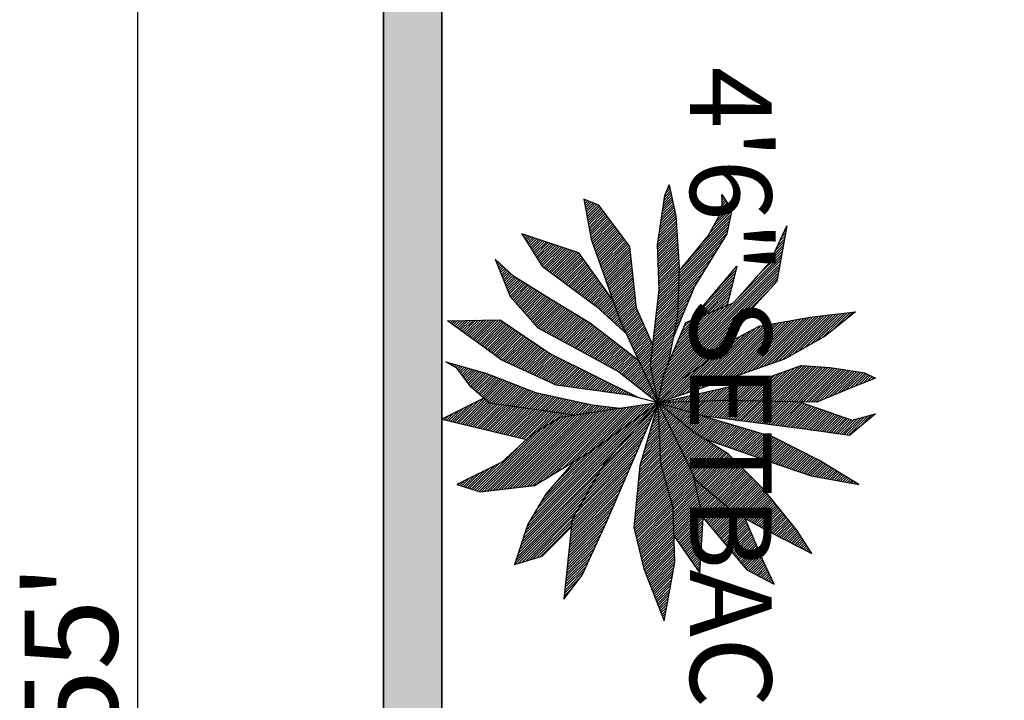
# Model space of a CAD drawing. Units: inches. Extents: x 3008 to 4088, y 1255 to 2137.
# Tile 6 of 30: x 3008 to 3093, y 1670 to 1728. Entities that reach past the tile are written whole.
import ezdxf

# ---------------------------------------------------------------- set-up
doc = ezdxf.new("R2010")
doc.units = ezdxf.units.IN
for name, color, linetype, lineweight in [('A-ANNO-DIMS', 2, 'Continuous', 18), ('A-ANNO-TEXT', 7, 'Continuous', 18), ('C-PROP', 1, 'Continuous', 35), ('C-PROP-PATT', 9, 'Continuous', 13), ('L-PLNT', 3, 'Continuous', 13), ('vfolhas', 114, 'Continuous', 5)]:
    doc.layers.add(name, color=color, linetype=linetype, lineweight=lineweight)
for name, color, linetype in [('vfolha', 72, 'Continuous'), ('vfolha2', 110, 'Continuous'), ('vfolhas2', 102, 'Continuous')]:
    doc.layers.add(name, color=color, linetype=linetype)
doc.styles.get("Standard").update_dxf_attribs({"font": 'arial.ttf'})
doc.dimstyles.new('ISO-25', dxfattribs={"dimtxt": 8, "dimasz": 2.5, "dimexe": 1.25, "dimexo": 0.625, "dimtad": 1, "dimdec": 1, "dimlunit": 3, "dimtxsty": 'Standard', "dimcen": 2.5, "dimadec": 0, "dimazin": 0, "dimtfac": 1, "dimtdec": 1, "dimtmove": 0, "dimatfit": 3, "dimfxl": 1, "dimarcsym": 0})
pattern_1 = [(45, (-2446.513311328918, 50.98607575111775), (-0.0044194173824159, 0.0044194173824159), [])]

# ---------------------------------------------------------------- blocks, each defined once
blk = doc.blocks.new('*D2')
at = {"layer": 'A-ANNO-DIMS', "color": 0, "lineweight": -2, "transparency": 16777216}
for p, q in [((3039.040660450281, 2003.966263701819), (3017.259837783714, 2003.966263701819)), ((3018.509837783714, 2001.466263701819), (3018.509837783714, 1346.466263701818)), ((3039.040660450281, 1343.966263701819), (3017.259837783714, 1343.966263701819))]:
    blk.add_line(p, q, dxfattribs=at)
at = {"layer": 'A-ANNO-DIMS', "color": 0, "transparency": 16777216}
for points in [[(3018.093171117048, 2001.466263701819), (3018.926504450381, 2001.466263701819), (3018.509837783714, 2003.966263701819)], [(3018.093171117048, 1346.466263701818), (3018.926504450381, 1346.466263701818), (3018.509837783714, 1343.966263701819)]]:
    blk.add_solid(points, dxfattribs=at)
at = {"layer": 'Defpoints', "color": 0, "transparency": 16777216}
for p in [(3039.665660450281, 2003.966263701819), (3018.509837783714, 1343.966263701819), (3039.665660450281, 1343.966263701819)]:
    blk.add_point(p, dxfattribs=at)
at = {"layer": 'A-ANNO-DIMS', "color": 0, "transparency": 16777216, "insert": (3013.816624959703, 1673.966263701817), "char_height": 8, "attachment_point": 5, "rotation": 90}
blk.add_mtext("55'", dxfattribs=at)
blk = doc.blocks.new('arbusto_PB_verde_grande')
at = {"layer": 'vfolha2'}
h = blk.add_hatch(dxfattribs=at)
h.set_pattern_fill('ANSI31', color=256, scale=0.05, style=0)
h.set_pattern_definition(pattern_1)
h.paths.add_polyline_path([(0.0294372067806137, 0.3565111995000905), (0.0002757213374309, 0.0904824516967153), (0.0262526469860234, -0.0393387531877068), (0.0469981892233875, 0.0623276281037022), (0.061889225542192, 0.09730735603225), (0.0937206571093441, 0.2657290609879511), (0.0995529541983444, 0.4347266728475463), (0.0878883600207985, 0.6131321160052893), (0.0644950804894791, 0.7226612468122938), (0.0498822921795466, 0.6850985919211043), (0.0236049096920681, 0.5129421461949732)])
h.paths.add_polyline_path([(0.3010556140521033, 0.4378855067140819), (0.1422506528203503, 0.2487134447506216), (0.266852050905866, 0.3002231891941697)])
h.paths.add_polyline_path([(0.3799518526907661, 0.2281664060967614), (0.23696550788001, 0.1519283823737274), (0.1842814899255529, 0.0936412855632796), (0.1112175483754357, 0.0435806358088371), (0.0262526469860234, -0.0393387531877068), (0.2806105286531701, 0.046670799373942), (0.368287258513679, 0.0779844568334922), (0.4675644913741336, 0.1123882778581162), (0.6106800891643901, 0.1937625850721077), (0.7158537102905315, 0.2782270558511755), (0.5581253241898877, 0.2594800635563387)])
h.paths.add_polyline_path([(0.5610094271460472, -0.2944145879103532), (0.7275183044680773, -0.3257282453699304), (0.5902350037659124, -0.2411951042894033), (0.4296225147095642, -0.1598207970754118), (0.0262526469860234, -0.0393387531877068), (0.1492236162166875, -0.1410738047805182), (0.188384525729089, -0.1660430415962635), (0.4150097263996438, -0.2443539381559163)])
h.paths.add_polyline_path([(-0.2742908800664451, -0.4477553710401593), (-0.3035164566863102, -0.7262821137067874), (-0.2392330063575799, -0.6417489726262603), (-0.1545685618070526, -0.4571632023383334), (0.0262526469860234, -0.0393387531877068), (-0.1632849618517582, -0.253761769454087)])
h.paths.add_polyline_path([(-0.5196319048504564, -0.2474441017210154), (-0.6773602909511, -0.3257282453699304), (-0.595579949356278, -0.3507242350964077), (-0.4057418836796105, -0.3288184089350068), (-0.2100715209143972, -0.2099501171312569), (0.0262526469860234, -0.0393387531877067), (-0.1487362647185048, -0.0659484949981665), (-0.3151810508638561, -0.0910131550261326), (-0.4145223749009972, -0.1504816360786947)])
h.paths.add_polyline_path([(-0.525464201939002, 0.2500722322581623), (-0.7094699705271239, 0.2469820686930859), (-0.5196319048504563, 0.1092981142930683), (-0.3297938391737886, 0.0216748096474362), (-0.0756723231683907, -0.012797681678677), (-0.0423442733277238, -0.0214762434946634), (-0.3502389245722667, 0.1312039404544406)])
h = blk.add_hatch(dxfattribs=at)
h.set_pattern_fill('ANSI31', color=256, scale=0.05, style=0)
h.set_pattern_definition(pattern_1)
h.paths.add_polyline_path([(-0.1896264355159187, 0.2970427184474999), (-0.0855343194014637, 0.2019191130931916), (-0.107846093921097, 0.2500722322581624), (-0.1320163779363008, 0.3186521089488384), (-0.2509616917118081, 0.4847873226019602), (-0.4495161574327255, 0.5505048010861913), (-0.3794645011925866, 0.437885506714082)])
h.paths.add_polyline_path([(0.0791078687994116, -0.4071025525838933), (0.0821399376597343, -0.5063128890747639), (0.1725528045713247, -0.635499975194648), (0.1842814899255529, -0.4415063736085472), (0.1490398072856009, -0.2917737067340336), (0.0262526469860234, -0.0393387531877068), (0.035269503869614, -0.253761769454087)])
at = {"layer": 'vfolhas'}
h = blk.add_hatch(dxfattribs=at)
h.set_pattern_fill('ANSI31', color=256, scale=0.05, style=0)
h.set_pattern_definition(pattern_1)
h.paths.add_polyline_path([(-0.0727882202122316, 0.506693148763361), (-0.180845944294532, 0.6506261005950194), (-0.2334007092690343, 0.6725319267564202), (-0.2071233267820105, 0.5317578087913261), (-0.1078460939210969, 0.2500722322581621), (0.0262526469860234, -0.0393387531877067), (0.0002757213374309, 0.0904824516967153), (0.0081597239746827, 0.1624051030085992), (-0.049394940681367, 0.2907937210158594)])
h.paths.add_polyline_path([(0.0990202003692698, 0.4192895091625076), (0.0937206571093441, 0.265729060987951), (0.0790571961243617, 0.1881439516147792), (0.1550559133052331, 0.3690091943633431), (0.2660618315199201, 0.5505048010861912), (0.2835587227860117, 0.6350379421667186), (0.2485008490776011, 0.6881887554862091), (0.2514490432099876, 0.6350379421667185), (0.2017783811911896, 0.5442558036545505)])
h.paths.add_polyline_path([(0.1229462337296639, 0.2407330712614737), (0.0469981892233875, 0.0623276281037022), (0.0262526469860234, -0.0393387531877067), (0.1112175483754356, 0.0435806358088371), (0.1842814899255529, 0.0936412855632796), (0.274778231564625, 0.1937625850721078), (0.3215006994505813, 0.2532310661246982), (0.4412871088866554, 0.3846660230931321), (0.4763449825955206, 0.5786596246792043), (0.4178938293553358, 0.4534736651424111), (0.289391019875012, 0.3095407133107528)])
h.paths.add_polyline_path([(0.581454512544525, -0.0377936714051543), (0.7070732190691449, 0.0153571419143647), (0.7859053665311252, 0.0466707993739419), (0.7479633898665554, 0.065486461970238), (0.6281769804304814, 0.0842334542651031), (0.5259515534371815, 0.0904824516967153), (0.3974487439568576, 0.0435806358088371), (0.0262526469860234, -0.0393387531877068), (0.2572813402989879, -0.0315446739735137), (0.4383389147538148, -0.034703507840078)])
h.paths.add_polyline_path([(0.5202160126333567, -0.0364714047610799), (0.438338914753814, -0.0347035078400779), (0.2572813402989879, -0.0315446739735137), (0.0262526469860234, -0.0393387531877068), (0.1796378832922042, -0.0851531985667382), (0.5376802387914114, -0.131665973482399), (0.6954086248920532, -0.1535717996437711), (0.785905366531125, -0.0785151601628513), (0.7041250249367578, -0.1004209863242522)])
h.paths.add_polyline_path([(0.2718941286089205, -0.2192892781280023), (0.1492236162166876, -0.1410738047805182), (0.0262526469860234, -0.0393387531877068), (0.1579400162613921, -0.3100714166401416), (0.2952233169635576, -0.4258495448787585), (0.4178938293553374, -0.4915670233629906), (0.5639576212784335, -0.5666923331453404), (0.5114028563039311, -0.4853180259313772), (0.3945646410006986, -0.3413850740996906)])
h.paths.add_polyline_path([(-0.0581754319022991, -0.4759101946332009), (-0.0231175581938885, -0.6198431464648595), (0.0469981892233875, -0.8013387531877071), (0.0849401658879572, -0.59793732030343), (0.0791078687994116, -0.4071025525838934), (0.035269503869614, -0.2537617694540871), (0.0262526469860234, -0.0393387531877068), (-0.037730346503821, -0.2600107668856992)])
h.paths.add_polyline_path([(-0.242181200490421, 0.1405431014511577), (-0.1107301968772561, 0.0685766255353144), (0.0262526469860234, -0.0393387531877067), (-0.0423455789620989, 0.1087094688700612), (-0.210071520914397, 0.2375742373949095), (-0.3648517128822022, 0.331446539472184), (-0.4787417340530456, 0.4034130153879689), (-0.5430251843817758, 0.4628814964405878), (-0.4904063282301365, 0.3314465394721821), (-0.394077289502519, 0.2219174086651207)])
h = blk.add_hatch(dxfattribs=at)
h.set_pattern_fill('ANSI31', color=256, scale=0.05, style=0)
h.set_pattern_definition(pattern_1)
h.paths.add_polyline_path([(-0.5721866698249584, 0.0623276281037022), (-0.7153022676152148, 0.1029804465599682), (-0.6773602909511, 0.0810746203985957), (-0.6276896289323022, 0.0153571419143646), (-0.5634702697802538, -0.0409525052716901), (-0.2646143236521083, -0.0833983906610745), (-0.1487362647185102, -0.0659484949981675), (-0.1015103002611421, -0.0587670644222552), (-0.2041751326491691, -0.0472015027033024), (-0.402793689546769, -0.0033898503805005)])
h.paths.add_polyline_path([(-0.5634702697802538, -0.0409525052716901), (-0.5827900422908869, -0.0240122930342424), (-0.7299150559256019, -0.0972621524577449), (-0.4334045373284922, -0.167900237669902), (-0.4145223749009971, -0.1504816360786947), (-0.3151810508638562, -0.0910131550261326), (-0.2646143236521083, -0.0833983906610745)])
h.paths.add_polyline_path([(-0.2769047876357005, -0.472666536023008), (-0.2742908800664452, -0.4477553710401595), (-0.1632849618517582, -0.253761769454087), (0.0262526469860233, -0.0393387531877068), (-0.2100715209143968, -0.2099501171312565), (-0.2672033595069225, -0.2446572846610163), (-0.3648517128821993, -0.35697323252802), (-0.4290710720342474, -0.4634121997699482), (-0.4758576310968862, -0.6042549880365016), (-0.3794645011925866, -0.576031494142029)])
h = blk.add_hatch(dxfattribs=at)
h.set_pattern_fill('ANSI31', color=256, scale=0.05, style=0)
h.set_pattern_definition(pattern_1)
h.paths.add_polyline_path([(0.3361134877609686, -0.6230019803313951), (0.4325066176652684, -0.6730626300858094), (0.3945646410006983, -0.5948471567383816), (0.3303002489141496, -0.4446410822727964), (0.2952233169635579, -0.4258495448787589), (0.1579400162613922, -0.3100714166401417), (0.1490398072856009, -0.2917737067340336), (0.184281489925553, -0.4415063736085473)])
at = {"layer": 'vfolha'}
for p, q in [((0.0262526469860234, -0.0393387531877068), (-0.148736264718508, -0.0659484949981675)), ((0.0262526469860234, -0.0393387531877068), (-0.037730346503821, -0.2600107668856992)), ((0.035269503869614, -0.253761769454087), (0.0262526469860234, -0.0393387531877068)), ((0.5202160126332558, -0.0364714047610448), (0.7041250249367579, -0.1004209863242522)), ((0.5376802387914097, -0.1316659734823986), (0.1796378832919174, -0.0851531985667009)), ((0.7859053665311251, -0.0785151601628513), (0.6954086248920534, -0.1535717996437711)), ((0.7041250249367579, -0.1004209863242522), (0.7859053665311251, -0.0785151601628513)), ((0.6954086248920534, -0.1535717996437711), (0.5376802387914097, -0.1316659734823986)), ((0.3945646410006986, -0.3413850740996906), (0.2718941286089205, -0.2192892781280022)), ((-0.2672033595067376, -0.2446572846608035), (-0.3648517128821993, -0.3569732325280199)), ((-0.037730346503821, -0.2600107668856992), (-0.0581754319022991, -0.475910194633201)), ((0.0791078687994116, -0.4071025525838934), (0.035269503869614, -0.253761769454087)), ((0.1579400162613922, -0.3100714166401417), (0.2952233169635576, -0.4258495448787585)), ((0.5114028563039313, -0.4853180259313774), (0.3945646410006986, -0.3413850740996906)), ((0.0849401658879572, -0.59793732030343), (0.0791078687994116, -0.4071025525838934)), ((0.2952233169635576, -0.4258495448787585), (0.4178938293553358, -0.4915670233629897)), ((0.4178938293553358, -0.4915670233629897), (0.5639576212784334, -0.5666923331453404)), ((0.5639576212784334, -0.5666923331453404), (0.5114028563039313, -0.4853180259313774)), ((0.0469981892233875, -0.8013387531877071), (0.0849401658879572, -0.59793732030343)), ((-0.0231175581938885, -0.6198431464648593), (0.0469981892233875, -0.8013387531877071))]:
    blk.add_line(p, q, dxfattribs=at)
at = {"layer": 'vfolha2'}
for p, q in [((0.0498822921795466, 0.6850985919211042), (0.0644950804894791, 0.7226612468122938)), ((0.0644950804894791, 0.7226612468122938), (0.0878883600207985, 0.6131321160052892)), ((0.0236049096920681, 0.5129421461949732), (0.0498822921795466, 0.6850985919211042)), ((0.0878883600207985, 0.6131321160052892), (0.0995529541983444, 0.4347266728475461)), ((-0.4495161574327256, 0.5505048010861913), (-0.3794645011925866, 0.4378855067140819)), ((-0.250961691711808, 0.4847873226019602), (-0.4495161574327256, 0.5505048010861913)), ((-0.1320163779364236, 0.31865210894901), (-0.250961691711808, 0.4847873226019602)), ((0.0294372067806137, 0.3565111995000905), (0.0236049096920681, 0.5129421461949732)), ((-0.3794645011925866, 0.4378855067140819), (-0.1896264355159189, 0.2970427184475)), ((0.0995529541983444, 0.4347266728475461), (0.0937206571093441, 0.265729060987951)), ((0.143391319128142, 0.2500722322581623), (0.3010556140521032, 0.4378855067140819)), ((0.3010556140521032, 0.4378855067140819), (0.2660618315199201, 0.2970427184475)), ((0.0002757213374309, 0.0904824516967153), (0.0294372067806137, 0.3565111995000905)), ((-0.1896264355159189, 0.2970427184475), (-0.0822034303200496, 0.1988752113042125)), ((0.5581253241898878, 0.2594800635563388), (0.7158537102905314, 0.2782270558511755)), ((0.7158537102905314, 0.2782270558511755), (0.61068008916439, 0.1937625850721076)), ((-0.7094699705271239, 0.2469820686930859), (-0.5254642019390019, 0.2500722322581623)), ((-0.5196319048504563, 0.1092981142930682), (-0.7094699705271239, 0.2469820686930859)), ((-0.5254642019390019, 0.2500722322581623), (-0.3502389245722668, 0.1312039404544407)), ((0.3799518526907661, 0.2281664060967614), (0.5581253241898878, 0.2594800635563388)), ((0.2369655078796597, 0.1519283823735407), (0.3799518526907661, 0.2281664060967614)), ((0.61068008916439, 0.1937625850721076), (0.4675644913741337, 0.1123882778581162)), ((-0.3297938391737887, 0.0216748096474362), (-0.5196319048504563, 0.1092981142930682)), ((-0.3502389245722668, 0.1312039404544407), (-0.0423442733276431, -0.0214762434947034)), ((0.0262526469860234, -0.0393387531877068), (0.0002757213374309, 0.0904824516967153)), ((0.3682872585136749, 0.0779844568334909), (0.2806105286531704, 0.0466707993739419)), ((0.2806105286531704, 0.0466707993739419), (0.0262526469860234, -0.0393387531877068)), ((-0.0756723231683907, -0.012797681678677), (-0.3297938391737887, 0.0216748096474362)), ((-0.148736264718508, -0.0659484949981675), (-0.3151810508638562, -0.0910131550261326)), ((-0.2100715209143971, -0.2099501171312568), (0.0262526469860234, -0.0393387531877068)), ((0.0262526469860234, -0.0393387531877068), (-0.1632849618517582, -0.253761769454087)), ((-0.1545685618070536, -0.4571632023383359), (0.0262526469860234, -0.0393387531877068)), ((0.4296225147095641, -0.1598207970754117), (0.0262526469860234, -0.0393387531877068)), ((0.0262526469860234, -0.0393387531877068), (0.1579400162613922, -0.3100714166401417)), ((-0.3151810508638562, -0.0910131550261326), (-0.4145223749009972, -0.1504816360786947)), ((-0.4145223749009972, -0.1504816360786947), (-0.5196319048504563, -0.2474441017210154)), ((0.1883845257293899, -0.1660430415963674), (0.4150097263996316, -0.2443539381559105)), ((0.5902350037659119, -0.2411951042894032), (0.4296225147095641, -0.1598207970754117)), ((-0.4057418836796103, -0.3288184089350068), (-0.2100715209143971, -0.2099501171312568)), ((-0.5196319048504563, -0.2474441017210154), (-0.6773602909511, -0.3257282453699304)), ((-0.1632849618517582, -0.253761769454087), (-0.2742908800664452, -0.4477553710401594)), ((0.4150097263996316, -0.2443539381559105), (0.5610094271460468, -0.294414587910353)), ((0.7275183044680773, -0.3257282453699304), (0.5902350037659119, -0.2411951042894032)), ((0.1842814899255529, -0.4415063736085472), (0.1490398072865275, -0.2917737067379704)), ((0.5610094271460468, -0.294414587910353), (0.7275183044680773, -0.3257282453699304)), ((-0.6773602909511, -0.3257282453699304), (-0.5955799493562779, -0.3507242350964077)), ((-0.5955799493562779, -0.3507242350964077), (-0.4057418836796103, -0.3288184089350068)), ((0.1725528045713247, -0.635499975194648), (0.1842814899255529, -0.4415063736085472)), ((-0.2742908800664452, -0.4477553710401594), (-0.3035164566863102, -0.7262821137067875)), ((0.0821399376596048, -0.5063128890745788), (0.1725528045713247, -0.635499975194648)), ((-0.3035164566863102, -0.7262821137067875), (-0.2392330063575798, -0.6417489726262602))]:
    blk.add_line(p, q, dxfattribs=at)
at = {"layer": 'vfolhas2'}
for p, q in [((-0.2334007092690342, 0.6725319267564203), (-0.2071233267820105, 0.5317578087913262)), ((-0.180845944294532, 0.6506261005950194), (-0.2334007092690342, 0.6725319267564203)), ((0.2514490432099876, 0.6350379421667185), (0.2485008490776011, 0.688188755486209)), ((0.2485008490776011, 0.688188755486209), (0.2835587227860117, 0.6350379421667185)), ((-0.0727882202122316, 0.5066931487633611), (-0.180845944294532, 0.6506261005950194)), ((0.2017783811911897, 0.5442558036545507), (0.2514490432099876, 0.6350379421667185)), ((0.2835587227860117, 0.6350379421667185), (0.2660618315199201, 0.5505048010861913)), ((0.4178938293553358, 0.4534736651424112), (0.4763449825955206, 0.5786596246792044)), ((0.4763449825955206, 0.5786596246792044), (0.4412871088866553, 0.384666023093132)), ((-0.2071233267820105, 0.5317578087913262), (-0.107846093921097, 0.2500722322581623)), ((0.0990202003690968, 0.4192895091622973), (0.2017783811911897, 0.5442558036545507)), ((0.2660618315199201, 0.5505048010861913), (0.1550559133052332, 0.3690091943633433)), ((-0.049394940681367, 0.2907937210158593), (-0.0727882202122316, 0.5066931487633611)), ((-0.5430251843817758, 0.4628814964405877), (-0.4904063282301366, 0.3314465394721822)), ((-0.4787417340530454, 0.4034130153879687), (-0.5430251843817758, 0.4628814964405877)), ((0.289391019875012, 0.3095407133107528), (0.4178938293553358, 0.4534736651424112)), ((-0.3648517128821993, 0.3314465394721822), (-0.4787417340530454, 0.4034130153879687)), ((0.4412871088866553, 0.384666023093132), (0.3215006994505813, 0.2532310661246981)), ((0.1550559133052332, 0.3690091943633433), (0.0779515085155538, 0.1855125853866468)), ((-0.4904063282301366, 0.3314465394721822), (-0.3940772895025191, 0.2219174086651208)), ((-0.2100715209143971, 0.2375742373949095), (-0.3648517128821993, 0.3314465394721822)), ((0.0081597239746145, 0.1624051030087514), (-0.049394940681367, 0.2907937210158593)), ((0.1229462337296638, 0.2407330712614737), (0.289391019875012, 0.3095407133107528)), ((-0.107846093921097, 0.2500722322581623), (0.0262526469860234, -0.0393387531877068)), ((0.0937206571093441, 0.265729060987951), (0.0618892255420462, 0.0973073560314788)), ((0.3215006994505813, 0.2532310661246981), (0.2747782315646248, 0.1937625850721076)), ((-0.3940772895025191, 0.2219174086651208), (-0.2421812004904211, 0.1405431014511578)), ((-0.0423455789618572, 0.1087094688698755), (-0.2100715209143971, 0.2375742373949095)), ((0.0469981892233875, 0.0623276281037022), (0.1229462337296638, 0.2407330712614737)), ((0.2747782315646248, 0.1937625850721076), (0.1842814899255529, 0.0936412855632796)), ((-0.2421812004904211, 0.1405431014511578), (-0.110730196877256, 0.0685766255353144)), ((0.4675644913741337, 0.1123882778581162), (0.3682872585136749, 0.0779844568334909)), ((-0.6773602909511, 0.0810746203985957), (-0.7153022676152148, 0.1029804465599682)), ((-0.7153022676152148, 0.1029804465599682), (-0.5721866698249585, 0.0623276281037022)), ((-0.627689628932302, 0.0153571419143646), (-0.6773602909511, 0.0810746203985957)), ((0.1842814899255529, 0.0936412855632796), (0.1112175483754356, 0.0435806358088371)), ((0.3974487439568577, 0.0435806358088371), (0.5259515534371815, 0.0904824516967153)), ((0.5259515534371815, 0.0904824516967153), (0.6281769804304816, 0.0842334542651031)), ((0.6281769804304816, 0.0842334542651031), (0.7479633898665555, 0.065486461970238)), ((-0.5721866698249585, 0.0623276281037022), (-0.402793689546769, -0.0033898503805005)), ((-0.110730196877256, 0.0685766255353144), (0.0262526469860234, -0.0393387531877068)), ((0.0262526469860234, -0.0393387531877068), (0.0469981892233875, 0.0623276281037022)), ((0.0262526469860234, -0.0393387531877068), (0.3974487439568577, 0.0435806358088371)), ((0.1112175483754356, 0.0435806358088371), (0.0262526469860234, -0.0393387531877068)), ((0.7859053665311251, 0.0466707993739419), (0.7070732190691446, 0.0153571419143646)), ((0.7479633898665555, 0.065486461970238), (0.7859053665311251, 0.0466707993739419)), ((-0.5634702697802539, -0.0409525052716902), (-0.627689628932302, 0.0153571419143646)), ((0.7070732190691446, 0.0153571419143646), (0.581454512544525, -0.0377936714051543)), ((-0.5827900422909523, -0.024012293034275), (-0.7299150559256021, -0.0972621524577449)), ((-0.402793689546769, -0.0033898503805005), (-0.2041751326491692, -0.0472015027033024)), ((0.0262526469860234, -0.0393387531877068), (-0.0756723231683907, -0.012797681678677)), ((0.257281340298988, -0.0315446739735137), (0.0262526469860234, -0.0393387531877068)), ((0.438338914753814, -0.0347035078400779), (0.257281340298988, -0.0315446739735137)), ((-0.2646143236520118, -0.0833983906610882), (-0.5634702697802539, -0.0409525052716902)), ((-0.2041751326491692, -0.0472015027033024), (-0.0983247256972106, -0.059125930826383)), ((0.1492236162166876, -0.1410738047805182), (0.0262526469860234, -0.0393387531877068)), ((0.581454512544525, -0.0377936714051543), (0.438338914753814, -0.0347035078400779)), ((-0.7299150559256021, -0.0972621524577449), (-0.4334045373288689, -0.1679002376698122)), ((0.2718941286089205, -0.2192892781280022), (0.1492236162166876, -0.1410738047805182)), ((-0.3648517128821993, -0.3569732325280199), (-0.4290710720342475, -0.4634121997699481)), ((0.1842814899255529, -0.4415063736085472), (0.3361134877609686, -0.6230019803313951)), ((0.3945646410006986, -0.594847156738382), (0.3290421606498342, -0.4417005347412868)), ((-0.4290710720342475, -0.4634121997699481), (-0.4758576310968863, -0.6042549880365016)), ((-0.3794645011925866, -0.5760314941420291), (-0.2769047876363118, -0.472666536023624)), ((-0.2392330063575798, -0.6417489726262602), (-0.1545685618070536, -0.4571632023383359)), ((-0.0581754319022991, -0.475910194633201), (-0.0231175581938885, -0.6198431464648593)), ((-0.4758576310968863, -0.6042549880365016), (-0.3794645011925866, -0.5760314941420291)), ((0.4325066176652684, -0.6730626300858092), (0.3945646410006986, -0.594847156738382)), ((0.3361134877609686, -0.6230019803313951), (0.4325066176652684, -0.6730626300858092))]:
    blk.add_line(p, q, dxfattribs=at)

msp = doc.modelspace()

# ---------------------------------------------------------------- hatches: boundary and pattern name
at = {"layer": 'C-PROP-PATT'}
h = msp.add_hatch(color=256, dxfattribs=at)
h.dxf.hatch_style = 1
h.paths.add_polyline_path([(3519.66566045028, 2003.966263701818), (3039.66566045028, 2003.966263701818), (3039.66566045028, 1343.966263701818), (3051.66566045028, 1343.966263701818), (3051.66566045028, 1348.966263701818), (3044.66566045028, 1348.966263701818), (3044.66566045028, 1998.966263701818), (3514.66566045028, 1998.966263701818), (3514.66566045028, 1348.966263701818), (3219.665660450281, 1348.966263701818), (3219.66566045028, 1343.966263701818), (3519.66566045028, 1343.966263701818)])

# ---------------------------------------------------------------- linework, layer by layer
at = {"layer": 'C-PROP'}
for p, q in [((3039.66566045028, 1343.966263701818), (3039.66566045028, 2003.966263701818)), ((3044.66566045028, 1348.966263701818), (3044.66566045028, 1998.966263701818))]:
    msp.add_line(p, q, dxfattribs=at)

# ---------------------------------------------------------------- block references
at = {"layer": 'L-PLNT', "xscale": 24.60366729364114, "yscale": 24.60366729364114, "zscale": 24.60366729364114}
msp.add_blockref('arbusto_PB_verde_grande', (3062.624247638893, 1696.378393485739), dxfattribs=at)

# ---------------------------------------------------------------- texts
at = {"layer": 'A-ANNO-TEXT', "insert": (3073.025924916954, 1724.30074670374), "char_height": 7, "attachment_point": 1, "rotation": 270}
msp.add_mtext_dynamic_manual_height_columns('{\\fTimes New Roman|b0|i0|c0|p18;4\'6" SETBACK}', width=105.6126751703486, gutter_width=12.5, heights=[0], dxfattribs=at)

# ---------------------------------------------------------------- dimensions: what is measured, and where the dimension line sits
at = {"layer": 'A-ANNO-DIMS'}
dim = msp.add_linear_dim(base=(3018.509837783714, 1343.966263701819), p1=(3039.66566045028, 2003.966263701818), p2=(3039.66566045028, 1343.966263701818), angle=90, dimstyle='ISO-25', override={"dimclrd": 0, "dimclre": 0, "dimclrt": 0}, dxfattribs=at)
dim.commit()
dim.dimension.update_dxf_attribs({"geometry": '*D2', "text_midpoint": (3013.816624959703, 1673.966263701817)})

doc.saveas('drawing.dxf')
